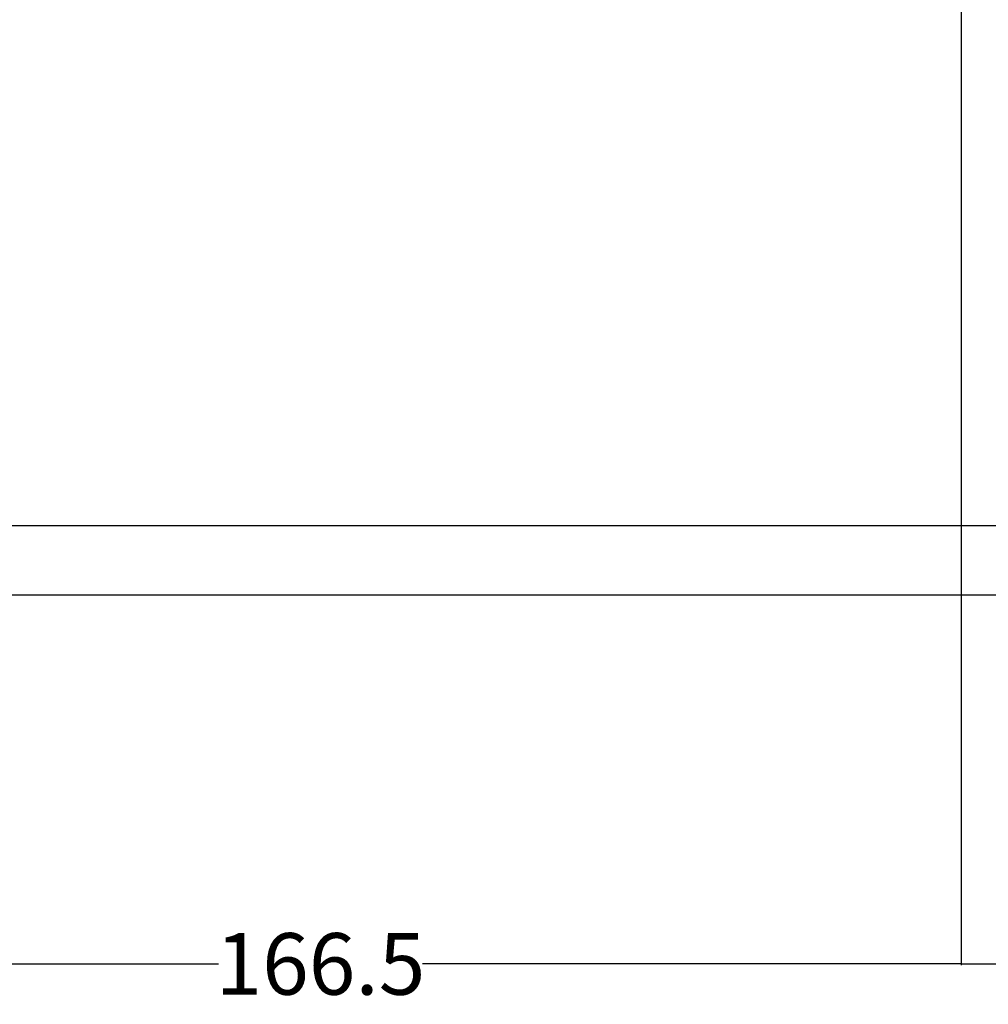
# Model space of a CAD drawing. Units: inches. Extents: x -48 to 50072, y 0 to 21068.
# Tile 22 of 75: x 341 to 467, y 161 to 289. Entities that reach past the tile are written whole.
import ezdxf

# ---------------------------------------------------------------- set-up
doc = ezdxf.new("R2010")
doc.units = ezdxf.units.IN
doc.header["$MEASUREMENT"] = 0
doc.layers.add('A-ANNO-DIMS', color=2, linetype='Continuous', lineweight=18)
doc.layers.add('C-PROP', color=7, linetype='Continuous', lineweight=25)
doc.styles.get("Standard").update_dxf_attribs({"font": 'arial.ttf'})
doc.dimstyles.get("Standard").update_dxf_attribs({"dimtxt": 8, "dimasz": 0.18, "dimexe": 0.18, "dimexo": 0.0625, "dimgap": 0.09, "dimtad": 0, "dimtih": 1, "dimtoh": 1, "dimdec": 1, "dimzin": 0, "dimdsep": 46, "dimlunit": 4, "dimtxsty": 'Standard', "dimblk": 'ARCHTICK', "dimcen": 0.09, "dimadec": 0, "dimazin": 0, "dimtfac": 1, "dimtdec": 1, "dimtofl": 0, "dimtmove": 0, "dimatfit": 3, "dimldrblk": 'ARCHTICK', "dimfxl": 1, "dimtolj": 1, "dimtzin": 0, "dimarcsym": 0})

# ---------------------------------------------------------------- blocks, each defined once
blk = doc.blocks.new('_ArchTick')
at = {"color": 0, "linetype": 'ByBlock', "const_width": 0.15}
blk.add_lwpolyline([(-0.5, -0.5), (0.5, 0.5)], dxfattribs=at)
blk = doc.blocks.new('*D118')
at = {"layer": 'A-ANNO-DIMS', "color": 0, "lineweight": -2, "transparency": 16777216}
for p, q in [((297.02, 488.71), (297.02, 165.94)), ((463.52, 488.71), (463.52, 165.94)), ((297.02, 166.12), (367.03, 166.12)), ((463.52, 166.12), (393.51, 166.12))]:
    blk.add_line(p, q, dxfattribs=at)
at = {"layer": 'Defpoints', "color": 0, "transparency": 16777216}
for p in [(297.02, 488.77), (463.52, 488.77), (463.52, 166.12)]:
    blk.add_point(p, dxfattribs=at)
at = {"layer": 'A-ANNO-DIMS', "color": 0, "lineweight": -2, "transparency": 16777216, "xscale": 0.18, "yscale": 0.18, "zscale": 0.18, "rotation": 180}
blk.add_blockref('_ArchTick', (297.02, 166.12), dxfattribs=at)
at = {"layer": 'A-ANNO-DIMS', "color": 0, "lineweight": -2, "transparency": 16777216, "xscale": 0.18, "yscale": 0.18, "zscale": 0.18}
blk.add_blockref('_ArchTick', (463.52, 166.12), dxfattribs=at)
at = {"layer": 'A-ANNO-DIMS', "color": 0, "transparency": 16777216, "insert": (380.27, 166.12), "char_height": 8, "attachment_point": 5}
blk.add_mtext('\\A1;166.5', dxfattribs=at)
blk = doc.blocks.new('*D119')
at = {"layer": 'A-ANNO-DIMS', "color": 0, "lineweight": -2, "transparency": 16777216}
for p, q in [((463.52, 451.01), (463.52, 165.94)), ((549.02, 451.01), (549.02, 165.94)), ((463.52, 166.12), (495.75, 166.12)), ((549.02, 166.12), (516.78, 166.12))]:
    blk.add_line(p, q, dxfattribs=at)
at = {"layer": 'Defpoints', "color": 0, "transparency": 16777216}
for p in [(463.52, 451.07), (549.02, 451.07), (549.02, 166.12)]:
    blk.add_point(p, dxfattribs=at)
at = {"layer": 'A-ANNO-DIMS', "color": 0, "lineweight": -2, "transparency": 16777216, "xscale": 0.18, "yscale": 0.18, "zscale": 0.18, "rotation": 180}
blk.add_blockref('_ArchTick', (463.52, 166.12), dxfattribs=at)
at = {"layer": 'A-ANNO-DIMS', "color": 0, "lineweight": -2, "transparency": 16777216, "xscale": 0.18, "yscale": 0.18, "zscale": 0.18}
blk.add_blockref('_ArchTick', (549.02, 166.12), dxfattribs=at)
at = {"layer": 'A-ANNO-DIMS', "color": 0, "transparency": 16777216, "insert": (506.27, 166.12), "char_height": 8, "attachment_point": 5}
blk.add_mtext('\\A1;85.5', dxfattribs=at)

msp = doc.modelspace()

# ---------------------------------------------------------------- linework, layer by layer
at = {"layer": 'C-PROP'}
for p, q in [((210.389, 223.075), (544.517, 223.075)), ((210.389, 214.075), (553.517, 214.075))]:
    msp.add_line(p, q, dxfattribs=at)

# ---------------------------------------------------------------- dimensions: what is measured, and where the dimension line sits
at = {"layer": 'A-ANNO-DIMS'}
for base, p1, p2, picture, middle in [((463.517, 166.125), (297.017, 488.775), (463.517, 488.775), '*D118', (380.267, 166.125)), ((549.017, 166.125), (463.517, 451.075), (549.017, 451.075), '*D119', (506.267, 166.125))]:
    dim = msp.add_linear_dim(base=base, p1=p1, p2=p2, dimstyle='Standard', override={"dimdec": 1, "dimlfac": 1, "dimrnd": 0, "dimzin": 0, "dimdsep": 46, "dimlunit": 2}, dxfattribs=at)
    dim.commit()
    dim.dimension.update_dxf_attribs({"geometry": picture, "text_midpoint": middle})

doc.saveas('drawing.dxf')
